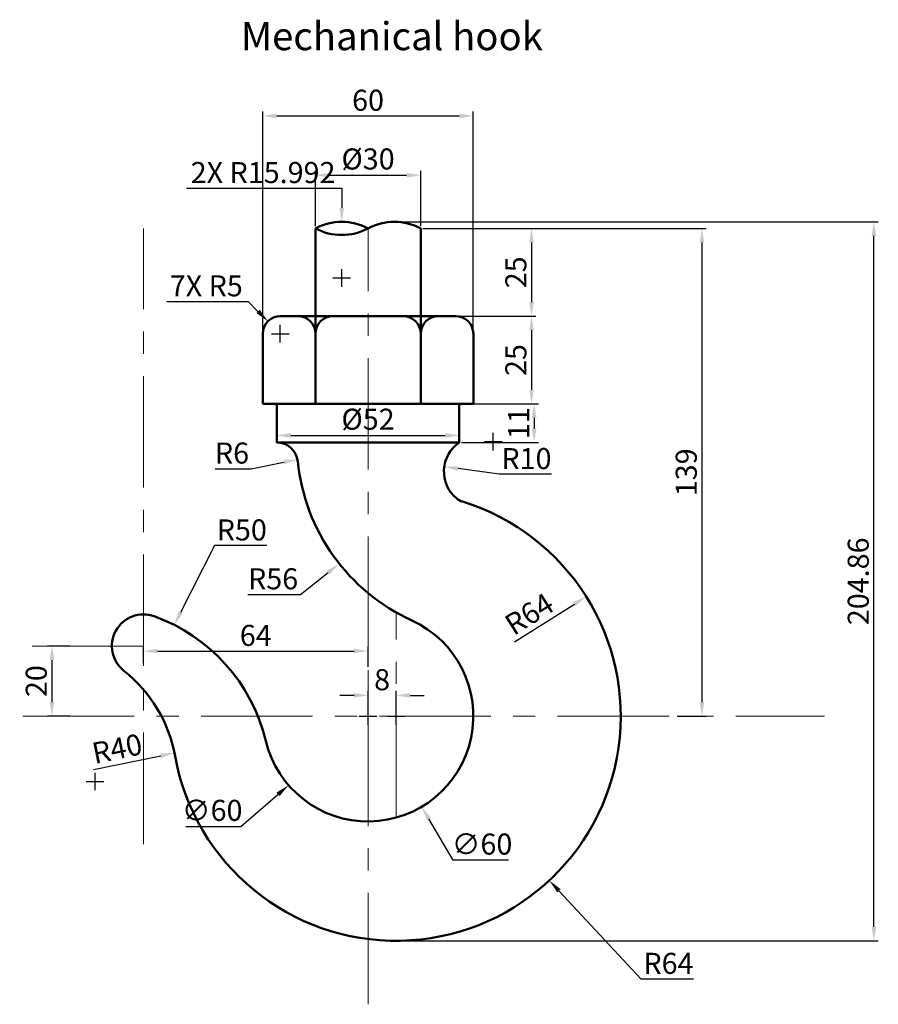
# Model space of a CAD drawing. Units: millimetres. Extents: x 42 to 286, y -15 to 266.
import ezdxf

# ---------------------------------------------------------------- set-up
doc = ezdxf.new("R2010")
doc.units = ezdxf.units.MM
doc.linetypes.add('CENTER', pattern=[50.8, 31.75, -6.35, 6.35, -6.35])
for name, color, linetype, lineweight in [('M-CNTR', 30, 'CENTER', 18), ('M-DIMS', 2, 'Continuous', 25), ('M-OUTL', 7, 'Continuous', 50), ('M-TEXT', 7, 'Continuous', 25)]:
    doc.layers.add(name, color=color, linetype=linetype, lineweight=lineweight)
doc.styles.get("Standard").update_dxf_attribs({"font": 'arial.ttf'})
doc.dimstyles.new('ISO-25', dxfattribs={"dimtxt": 6, "dimasz": 4, "dimexe": 1.25, "dimexo": 0.625, "dimtad": 1, "dimtoh": 1, "dimdec": 1, "dimtxsty": 'Standard', "dimcen": 2.5, "dimadec": 0, "dimazin": 0, "dimtfac": 1, "dimtdec": 1, "dimtofl": 0, "dimtmove": 0, "dimatfit": 3, "dimfxl": 1, "dimarcsym": 0})

# ---------------------------------------------------------------- blocks, each defined once
blk = doc.blocks.new('*D1')
at = {"layer": 'Defpoints', "color": 0, "transparency": 16777216}
for p in [(155.92, 206.24), (228.34, 67.24), (236.06, 67.24)]:
    blk.add_point(p, dxfattribs=at)
at = {"layer": 'M-DIMS', "color": 0, "lineweight": -2, "transparency": 16777216}
for p, q in [((156.55, 206.24), (237.31, 206.24)), ((236.06, 202.24), (236.06, 71.24)), ((228.97, 67.24), (237.31, 67.24))]:
    blk.add_line(p, q, dxfattribs=at)
at = {"layer": 'M-DIMS', "color": 0, "transparency": 16777216}
for points in [[(235.39, 202.24), (236.73, 202.24), (236.06, 206.24)], [(235.39, 71.24), (236.73, 71.24), (236.06, 67.24)]]:
    blk.add_solid(points, dxfattribs=at)
at = {"layer": 'M-DIMS', "color": 0, "transparency": 16777216, "insert": (232.37, 136.74), "char_height": 6, "attachment_point": 5, "rotation": 90}
blk.add_mtext('139', dxfattribs=at)
blk = doc.blocks.new('*D2')
at = {"layer": 'Defpoints', "color": 0, "transparency": 16777216}
for p in [(56.56, 87.24), (50.84, 67.24), (56.56, 67.24)]:
    blk.add_point(p, dxfattribs=at)
at = {"layer": 'M-DIMS', "color": 0, "lineweight": -2, "transparency": 16777216}
for p, q in [((55.94, 87.24), (49.59, 87.24)), ((50.84, 83.24), (50.84, 71.24)), ((55.94, 67.24), (49.59, 67.24))]:
    blk.add_line(p, q, dxfattribs=at)
at = {"layer": 'M-DIMS', "color": 0, "transparency": 16777216}
for points in [[(50.17, 83.24), (51.51, 83.24), (50.84, 87.24)], [(50.17, 71.24), (51.51, 71.24), (50.84, 67.24)]]:
    blk.add_solid(points, dxfattribs=at)
at = {"layer": 'M-DIMS', "color": 0, "transparency": 16777216, "insert": (47.15, 77.24), "char_height": 6, "attachment_point": 5, "rotation": 90}
blk.add_mtext('20', dxfattribs=at)
blk = doc.blocks.new('*D3')
at = {"layer": 'Defpoints', "color": 0, "transparency": 16777216}
for p in [(148.92, 73.18), (140.92, 67.24), (148.92, 67.24)]:
    blk.add_point(p, dxfattribs=at)
at = {"layer": 'M-DIMS', "color": 0, "lineweight": -2, "transparency": 16777216}
for p, q in [((136.92, 73.18), (132.92, 73.18)), ((140.92, 67.87), (140.92, 74.43)), ((148.92, 67.87), (148.92, 74.43)), ((152.92, 73.18), (156.92, 73.18))]:
    blk.add_line(p, q, dxfattribs=at)
at = {"layer": 'M-DIMS', "color": 0, "transparency": 16777216}
for points in [[(136.92, 73.85), (136.92, 72.52), (140.92, 73.18)], [(152.92, 73.85), (152.92, 72.52), (148.92, 73.18)]]:
    blk.add_solid(points, dxfattribs=at)
at = {"layer": 'M-DIMS', "color": 0, "transparency": 16777216, "insert": (144.92, 76.87), "char_height": 6, "attachment_point": 5}
blk.add_mtext('8', dxfattribs=at)
blk = doc.blocks.new('*D4')
at = {"layer": 'Defpoints', "color": 0, "transparency": 16777216}
for p in [(166.92, 156.24), (166.92, 145.24), (188.25, 145.24)]:
    blk.add_point(p, dxfattribs=at)
at = {"layer": 'M-DIMS', "color": 0, "lineweight": -2, "transparency": 16777216}
for p, q in [((167.55, 156.24), (189.5, 156.24)), ((188.25, 152.24), (188.25, 149.24)), ((167.55, 145.24), (189.5, 145.24))]:
    blk.add_line(p, q, dxfattribs=at)
at = {"layer": 'M-DIMS', "color": 0, "transparency": 16777216}
for points in [[(187.59, 152.24), (188.92, 152.24), (188.25, 156.24)], [(187.59, 149.24), (188.92, 149.24), (188.25, 145.24)]]:
    blk.add_solid(points, dxfattribs=at)
at = {"layer": 'M-DIMS', "color": 0, "transparency": 16777216, "insert": (184.62, 150.74), "char_height": 6, "attachment_point": 5, "rotation": 90}
blk.add_mtext('11', dxfattribs=at)
blk = doc.blocks.new('*D5')
at = {"layer": 'Defpoints', "color": 0, "transparency": 16777216}
for p in [(155.92, 181.24), (170.92, 156.24), (187.5, 156.24)]:
    blk.add_point(p, dxfattribs=at)
at = {"layer": 'M-DIMS', "color": 0, "lineweight": -2, "transparency": 16777216}
for p, q in [((156.55, 181.24), (188.75, 181.24)), ((187.5, 177.24), (187.5, 160.24)), ((171.55, 156.24), (188.75, 156.24))]:
    blk.add_line(p, q, dxfattribs=at)
at = {"layer": 'M-DIMS', "color": 0, "transparency": 16777216}
for points in [[(186.84, 177.24), (188.17, 177.24), (187.5, 181.24)], [(186.84, 160.24), (188.17, 160.24), (187.5, 156.24)]]:
    blk.add_solid(points, dxfattribs=at)
at = {"layer": 'M-DIMS', "color": 0, "transparency": 16777216, "insert": (183.82, 168.74), "char_height": 6, "attachment_point": 5, "rotation": 90}
blk.add_mtext('25', dxfattribs=at)
blk = doc.blocks.new('*D6')
at = {"layer": 'Defpoints', "color": 0, "transparency": 16777216}
for p in [(155.92, 206.24), (165.92, 181.24), (187.5, 181.24)]:
    blk.add_point(p, dxfattribs=at)
at = {"layer": 'M-DIMS', "color": 0, "lineweight": -2, "transparency": 16777216}
for p, q in [((156.55, 206.24), (188.75, 206.24)), ((187.5, 202.24), (187.5, 185.24)), ((166.55, 181.24), (188.75, 181.24))]:
    blk.add_line(p, q, dxfattribs=at)
at = {"layer": 'M-DIMS', "color": 0, "transparency": 16777216}
for points in [[(186.84, 202.24), (188.17, 202.24), (187.5, 206.24)], [(186.84, 185.24), (188.17, 185.24), (187.5, 181.24)]]:
    blk.add_solid(points, dxfattribs=at)
at = {"layer": 'M-DIMS', "color": 0, "transparency": 16777216, "insert": (183.82, 193.74), "char_height": 6, "attachment_point": 5, "rotation": 90}
blk.add_mtext('25', dxfattribs=at)
blk = doc.blocks.new('*D7')
at = {"layer": 'Defpoints', "color": 0, "transparency": 16777216}
for p in [(170.92, 238.3), (110.92, 156.24), (170.92, 156.24)]:
    blk.add_point(p, dxfattribs=at)
at = {"layer": 'M-DIMS', "color": 0, "lineweight": -2, "transparency": 16777216}
for p, q in [((110.92, 156.87), (110.92, 239.55)), ((170.92, 156.87), (170.92, 239.55)), ((114.92, 238.3), (166.92, 238.3))]:
    blk.add_line(p, q, dxfattribs=at)
at = {"layer": 'M-DIMS', "color": 0, "transparency": 16777216}
for points in [[(114.92, 238.97), (114.92, 237.63), (110.92, 238.3)], [(166.92, 238.97), (166.92, 237.63), (170.92, 238.3)]]:
    blk.add_solid(points, dxfattribs=at)
at = {"layer": 'M-DIMS', "color": 0, "transparency": 16777216, "insert": (140.92, 241.99), "char_height": 6, "attachment_point": 5}
blk.add_mtext('60', dxfattribs=at)
blk = doc.blocks.new('*D8')
at = {"layer": 'Defpoints', "color": 0, "transparency": 16777216}
for p in [(155.92, 221.41), (125.92, 206.24), (155.92, 206.24)]:
    blk.add_point(p, dxfattribs=at)
at = {"layer": 'M-DIMS', "color": 0, "lineweight": -2, "transparency": 16777216}
for p, q in [((125.92, 206.87), (125.92, 222.66)), ((155.92, 206.87), (155.92, 222.66)), ((129.92, 221.41), (151.92, 221.41))]:
    blk.add_line(p, q, dxfattribs=at)
at = {"layer": 'M-DIMS', "color": 0, "transparency": 16777216}
for points in [[(129.92, 222.07), (129.92, 220.74), (125.92, 221.41)], [(151.92, 222.07), (151.92, 220.74), (155.92, 221.41)]]:
    blk.add_solid(points, dxfattribs=at)
at = {"layer": 'M-DIMS', "color": 0, "transparency": 16777216, "insert": (140.92, 225.26), "char_height": 6, "attachment_point": 5}
blk.add_mtext('%%C30', dxfattribs=at)
blk = doc.blocks.new('*D9')
at = {"layer": 'Defpoints', "color": 0, "transparency": 16777216}
for p in [(114.92, 150.74), (166.92, 150.74), (166.92, 147.25)]:
    blk.add_point(p, dxfattribs=at)
at = {"layer": 'M-DIMS', "color": 0, "lineweight": -2, "transparency": 16777216}
for p, q in [((114.92, 150.12), (114.92, 146)), ((166.92, 150.12), (166.92, 146)), ((118.92, 147.25), (162.92, 147.25))]:
    blk.add_line(p, q, dxfattribs=at)
at = {"layer": 'M-DIMS', "color": 0, "transparency": 16777216}
for points in [[(118.92, 147.92), (118.92, 146.58), (114.92, 147.25)], [(162.92, 147.92), (162.92, 146.58), (166.92, 147.25)]]:
    blk.add_solid(points, dxfattribs=at)
at = {"layer": 'M-DIMS', "color": 0, "transparency": 16777216, "insert": (140.92, 151.1), "char_height": 6, "attachment_point": 5}
blk.add_mtext('%%C52', dxfattribs=at)
blk = doc.blocks.new('*D10')
at = {"layer": 'Defpoints', "color": 0, "transparency": 16777216}
for p in [(120.8, 140.43), (114.92, 139.24)]:
    blk.add_point(p, dxfattribs=at)
at = {"layer": 'M-DIMS', "color": 0, "lineweight": -2, "transparency": 16777216}
for p, q in [((97.31, 137.76), (107.61, 137.76)), ((107.61, 137.76), (116.88, 139.64))]:
    blk.add_line(p, q, dxfattribs=at)
at = {"layer": 'M-DIMS', "color": 0, "transparency": 16777216}
blk.add_solid([(116.75, 140.29), (117.02, 138.98), (120.8, 140.43)], dxfattribs=at)
at = {"layer": 'M-DIMS', "color": 0, "transparency": 16777216, "insert": (102.15, 141.45), "char_height": 6, "attachment_point": 5}
blk.add_mtext('R6', dxfattribs=at)
blk = doc.blocks.new('*D11')
at = {"layer": 'Defpoints', "color": 0, "transparency": 16777216}
for p in [(162.64, 138.34), (172.54, 136.98)]:
    blk.add_point(p, dxfattribs=at)
at = {"layer": 'M-DIMS', "color": 0, "lineweight": -2, "transparency": 16777216}
for p, q in [((178.27, 136.2), (166.6, 137.8)), ((193.21, 136.2), (178.27, 136.2))]:
    blk.add_line(p, q, dxfattribs=at)
at = {"layer": 'M-DIMS', "color": 0, "transparency": 16777216}
blk.add_solid([(166.69, 138.46), (166.51, 137.14), (162.64, 138.34)], dxfattribs=at)
at = {"layer": 'M-DIMS', "color": 0, "transparency": 16777216, "insert": (186.06, 139.88), "char_height": 6, "attachment_point": 5}
blk.add_mtext('R10', dxfattribs=at)
blk = doc.blocks.new('*D12')
at = {"layer": 'Defpoints', "color": 0, "transparency": 16777216}
for p in [(176.61, 145.49), (132.72, 110.7)]:
    blk.add_point(p, dxfattribs=at)
at = {"layer": 'M-DIMS', "color": 0, "lineweight": -2, "transparency": 16777216}
for p, q in [((176.61, 142.99), (176.61, 147.99)), ((174.11, 145.49), (179.11, 145.49)), ((121.65, 101.93), (129.59, 108.22)), ((106.69, 101.93), (121.65, 101.93))]:
    blk.add_line(p, q, dxfattribs=at)
at = {"layer": 'M-DIMS', "color": 0, "transparency": 16777216}
blk.add_solid([(129.17, 108.74), (130, 107.7), (132.72, 110.7)], dxfattribs=at)
at = {"layer": 'M-DIMS', "color": 0, "transparency": 16777216, "insert": (113.86, 105.62), "char_height": 6, "attachment_point": 5}
blk.add_mtext('R56', dxfattribs=at)
blk = doc.blocks.new('*D13')
at = {"layer": 'Defpoints', "color": 0, "transparency": 16777216}
for p in [(203.09, 101.33), (148.92, 67.24)]:
    blk.add_point(p, dxfattribs=at)
at = {"layer": 'M-DIMS', "color": 0, "lineweight": -2, "transparency": 16777216}
blk.add_line((182.65, 88.46), (199.71, 99.2), dxfattribs=at)
at = {"layer": 'M-DIMS', "color": 0, "transparency": 16777216}
blk.add_solid([(199.35, 99.76), (200.06, 98.63), (203.09, 101.33)], dxfattribs=at)
at = {"layer": 'M-DIMS', "color": 0, "transparency": 16777216, "insert": (187.27, 95.73), "char_height": 6, "attachment_point": 5, "rotation": 32.1817}
blk.add_mtext('R64', dxfattribs=at)
blk = doc.blocks.new('*D14')
at = {"layer": 'Defpoints', "color": 0, "transparency": 16777216}
for p in [(85.77, 56.79), (46.58, 48.77)]:
    blk.add_point(p, dxfattribs=at)
at = {"layer": 'M-DIMS', "color": 0, "lineweight": -2, "transparency": 16777216}
blk.add_line((62.68, 52.06), (81.85, 55.98), dxfattribs=at)
at = {"layer": 'M-DIMS', "color": 0, "transparency": 16777216}
blk.add_solid([(81.71, 56.64), (81.98, 55.33), (85.77, 56.79)], dxfattribs=at)
at = {"layer": 'M-DIMS', "color": 0, "transparency": 16777216, "insert": (69.56, 57.24), "char_height": 6, "attachment_point": 5, "rotation": 11.5627}
blk.add_mtext('R40', dxfattribs=at)
blk = doc.blocks.new('*D15')
at = {"layer": 'Defpoints', "color": 0, "transparency": 16777216}
for p in [(85.7, 93.24), (63.12, 48.64)]:
    blk.add_point(p, dxfattribs=at)
at = {"layer": 'M-DIMS', "color": 0, "lineweight": -2, "transparency": 16777216}
for p, q in [((97.15, 115.86), (87.51, 96.81)), ((112.09, 115.86), (97.15, 115.86)), ((63.12, 46.14), (63.12, 51.14)), ((60.62, 48.64), (65.62, 48.64))]:
    blk.add_line(p, q, dxfattribs=at)
at = {"layer": 'M-DIMS', "color": 0, "transparency": 16777216}
blk.add_solid([(86.91, 97.11), (88.1, 96.51), (85.7, 93.24)], dxfattribs=at)
at = {"layer": 'M-DIMS', "color": 0, "transparency": 16777216, "insert": (104.94, 119.55), "char_height": 6, "attachment_point": 5}
blk.add_mtext('R50', dxfattribs=at)
blk = doc.blocks.new('*D16')
at = {"layer": 'Defpoints', "color": 0, "transparency": 16777216}
for p in [(125.65, 93.06), (156.2, 41.42)]:
    blk.add_point(p, dxfattribs=at)
at = {"layer": 'M-DIMS', "color": 0, "lineweight": -2, "transparency": 16777216}
for p, q in [((140.92, 64.74), (140.92, 69.74)), ((138.42, 67.24), (143.42, 67.24)), ((165.22, 26.17), (158.24, 37.98)), ((180.95, 26.17), (165.22, 26.17))]:
    blk.add_line(p, q, dxfattribs=at)
at = {"layer": 'M-DIMS', "color": 0, "transparency": 16777216}
blk.add_solid([(158.81, 38.32), (157.66, 37.64), (156.2, 41.42)], dxfattribs=at)
at = {"layer": 'M-DIMS', "color": 0, "transparency": 16777216, "insert": (173.4, 30.03), "char_height": 6, "attachment_point": 5}
blk.add_mtext('∅60', dxfattribs=at)
blk = doc.blocks.new('*D17')
at = {"layer": 'Defpoints', "color": 0, "transparency": 16777216}
for p in [(140.92, 85.8), (76.92, 81.77), (140.92, 80.64)]:
    blk.add_point(p, dxfattribs=at)
at = {"layer": 'M-DIMS', "color": 0, "lineweight": -2, "transparency": 16777216}
for p, q in [((76.92, 82.4), (76.92, 87.05)), ((140.92, 81.27), (140.92, 87.05)), ((80.92, 85.8), (136.92, 85.8))]:
    blk.add_line(p, q, dxfattribs=at)
at = {"layer": 'M-DIMS', "color": 0, "transparency": 16777216}
for points in [[(80.92, 86.47), (80.92, 85.14), (76.92, 85.8)], [(136.92, 86.47), (136.92, 85.14), (140.92, 85.8)]]:
    blk.add_solid(points, dxfattribs=at)
at = {"layer": 'M-DIMS', "color": 0, "transparency": 16777216, "insert": (108.92, 89.49), "char_height": 6, "attachment_point": 5}
blk.add_mtext('64', dxfattribs=at)
blk = doc.blocks.new('*D18')
at = {"layer": 'Defpoints', "color": 0, "transparency": 16777216}
for p in [(148.42, 208.11), (285.08, 208.11), (150.14, 3.25)]:
    blk.add_point(p, dxfattribs=at)
at = {"layer": 'M-DIMS', "color": 0, "lineweight": -2, "transparency": 16777216}
for p, q in [((149.05, 208.11), (286.33, 208.11)), ((285.08, 7.25), (285.08, 204.11)), ((150.76, 3.25), (286.33, 3.25))]:
    blk.add_line(p, q, dxfattribs=at)
at = {"layer": 'M-DIMS', "color": 0, "transparency": 16777216}
for points in [[(284.41, 204.11), (285.74, 204.11), (285.08, 208.11)], [(284.41, 7.25), (285.74, 7.25), (285.08, 3.25)]]:
    blk.add_solid(points, dxfattribs=at)
at = {"layer": 'M-DIMS', "color": 0, "transparency": 16777216, "insert": (281.39, 105.68), "char_height": 6, "attachment_point": 5, "rotation": 90}
blk.add_mtext('204.86', dxfattribs=at)
blk = doc.blocks.new('*D19')
at = {"layer": 'Defpoints', "color": 0, "transparency": 16777216}
for p in [(148.92, 67.24), (192.57, 20.43)]:
    blk.add_point(p, dxfattribs=at)
at = {"layer": 'M-DIMS', "color": 0, "lineweight": -2, "transparency": 16777216}
for p, q in [((148.92, 64.74), (148.92, 69.74)), ((146.42, 67.24), (151.42, 67.24)), ((218.75, -7.66), (195.29, 17.5)), ((233.69, -7.66), (218.75, -7.66))]:
    blk.add_line(p, q, dxfattribs=at)
at = {"layer": 'M-DIMS', "color": 0, "transparency": 16777216}
blk.add_solid([(195.78, 17.96), (194.81, 17.05), (192.57, 20.43)], dxfattribs=at)
at = {"layer": 'M-DIMS', "color": 0, "transparency": 16777216, "insert": (226.53, -3.97), "char_height": 6, "attachment_point": 5}
blk.add_mtext('R64', dxfattribs=at)
blk = doc.blocks.new('*D20')
at = {"layer": 'Defpoints', "color": 0, "transparency": 16777216}
for p in [(163.58, 86.91), (118.27, 47.57)]:
    blk.add_point(p, dxfattribs=at)
at = {"layer": 'M-DIMS', "color": 0, "lineweight": -2, "transparency": 16777216}
for p, q in [((140.92, 64.74), (140.92, 69.74)), ((138.42, 67.24), (143.42, 67.24)), ((104.68, 35.77), (115.25, 44.95)), ((88.95, 35.77), (104.68, 35.77))]:
    blk.add_line(p, q, dxfattribs=at)
at = {"layer": 'M-DIMS', "color": 0, "transparency": 16777216}
blk.add_solid([(114.81, 45.45), (115.69, 44.45), (118.27, 47.57)], dxfattribs=at)
at = {"layer": 'M-DIMS', "color": 0, "transparency": 16777216, "insert": (96.5, 39.63), "char_height": 6, "attachment_point": 5}
blk.add_mtext('∅60', dxfattribs=at)
blk = doc.blocks.new('*D21')
at = {"layer": 'Defpoints', "color": 0, "transparency": 16777216}
for p in [(133.42, 208.11), (133.42, 192.12)]:
    blk.add_point(p, dxfattribs=at)
at = {"layer": 'M-DIMS', "color": 0, "lineweight": -2, "transparency": 16777216}
for p, q in [((89.21, 217.7), (133.42, 217.7)), ((133.42, 217.7), (133.42, 212.11)), ((133.42, 189.62), (133.42, 194.62)), ((130.92, 192.12), (135.92, 192.12))]:
    blk.add_line(p, q, dxfattribs=at)
at = {"layer": 'M-DIMS', "color": 0, "transparency": 16777216}
blk.add_solid([(134.09, 212.11), (132.76, 212.11), (133.42, 208.11)], dxfattribs=at)
at = {"layer": 'M-DIMS', "color": 0, "transparency": 16777216, "insert": (111.01, 221.39), "char_height": 6, "attachment_point": 5}
blk.add_mtext('2X R15.992', dxfattribs=at)
blk = doc.blocks.new('*D22')
at = {"layer": 'Defpoints', "color": 0, "transparency": 16777216}
for p in [(112.39, 179.78), (115.92, 176.24)]:
    blk.add_point(p, dxfattribs=at)
at = {"layer": 'M-DIMS', "color": 0, "lineweight": -2, "transparency": 16777216}
for p, q in [((83.54, 185.43), (106.73, 185.43)), ((106.73, 185.43), (109.56, 182.6)), ((115.92, 173.74), (115.92, 178.74)), ((113.42, 176.24), (118.42, 176.24))]:
    blk.add_line(p, q, dxfattribs=at)
at = {"layer": 'M-DIMS', "color": 0, "transparency": 16777216}
blk.add_solid([(110.03, 183.08), (109.09, 182.13), (112.39, 179.78)], dxfattribs=at)
at = {"layer": 'M-DIMS', "color": 0, "transparency": 16777216, "insert": (94.82, 189.11), "char_height": 6, "attachment_point": 5}
blk.add_mtext('7X R5', dxfattribs=at)

msp = doc.modelspace()

# ---------------------------------------------------------------- linework, layer by layer
at = {"layer": 'M-CNTR'}
for p, q in [((76.9233, 30.8034), (76.9233, 206.2406)), ((140.9233, -14.8615), (140.9233, 206.2406)), ((148.9233, 38.327), (148.9233, 96.8096)), ((76.9233, 87.2406), (41.6504, 87.2406)), ((42.5381, 67.2406), (270.977, 67.2406))]:
    msp.add_line(p, q, dxfattribs=at)
at = {"layer": 'M-OUTL'}
for p, q in [((125.9233, 156.2406), (125.9233, 206.2406)), ((155.9233, 206.2406), (155.9233, 156.2406)), ((115.9233, 181.2406), (165.9233, 181.2406)), ((110.9233, 156.2406), (110.9233, 176.2406)), ((170.9233, 176.2406), (170.9233, 156.2406)), ((170.9233, 156.2406), (110.9233, 156.2406))]:
    msp.add_line(p, q, dxfattribs=at)
msp.add_lwpolyline([(114.9233, 156.2406), (166.9233, 156.2406), (166.9233, 145.2406), (114.9233, 145.2406)], close=True, dxfattribs=at)
for centre, radius, start, end in [((133.4233, 192.1163), 15.9921, 62.031765, 117.968235), ((148.4233, 192.1163), 15.9921, 62.031765, 117.968235), ((133.4233, 220.365), 15.9921, 242.031765, 297.968235), ((115.9233, 176.2406), 5, 90, 180), ((120.9233, 176.2406), 5, 0, 90), ((130.9233, 176.2406), 5, 90, 180), ((150.9233, 176.2406), 5, 0, 90), ((160.9233, 176.2406), 5, 90, 180), ((165.9233, 176.2406), 5, 0, 90), ((114.9233, 139.2406), 6, 5.78298, 90), ((172.5438, 136.9808), 10, 124.197644, 229.903617), ((176.6078, 145.4878), 56, 185.78298, 245.484738), ((169.3234, 133.156), 5, 229.903617, 252.80325), ((148.9233, 67.2406), 64, 190.230905, 72.80325), ((76.9233, 87.2406), 9, 70.321528, 231.733931), ((63.1169, 48.6351), 50, 13.448339, 70.321528), ((140.9233, 67.2406), 30, 193.448339, 65.484738), ((46.5769, 48.7686), 40, 10.230905, 51.733931)]:
    msp.add_arc(centre, radius, start, end, dxfattribs=at)

# ---------------------------------------------------------------- texts
at = {"layer": 'M-TEXT', "insert": (104.7025, 265.0387), "char_height": 8, "attachment_point": 1}
msp.add_mtext_dynamic_manual_height_columns('Mechanical hook', width=86.743585, gutter_width=12.5, heights=[0], dxfattribs=at)

# ---------------------------------------------------------------- dimensions: what is measured, and where the dimension line sits
at = {"layer": 'M-DIMS'}
for base, p1, p2, picture, middle in [((170.9233, 238.2993), (110.9233, 156.2406), (170.9233, 156.2406), '*D7', (140.9233, 241.9877)), ((140.9233, 85.8037), (76.9233, 81.7723), (140.9233, 80.6435), '*D17', (108.9233, 89.4921)), ((148.9233, 73.1818), (140.9233, 67.2406), (148.9233, 67.2406), '*D3', (144.9233, 76.8702))]:
    dim = msp.add_linear_dim(base=base, p1=p1, p2=p2, dimstyle='ISO-25', override={"dimclrd": 0, "dimclre": 0, "dimclrt": 0}, dxfattribs=at)
    dim.commit()
    dim.dimension.update_dxf_attribs({"geometry": picture, "text_midpoint": middle})
dim = msp.add_radius_dim(center=(133.4233, 192.1163), mpoint=(133.423, 208.1084), text='2X <>', dimstyle='ISO-25', override={"dimdec": 3, "dimlfac": 1, "dimrnd": 0, "dimzin": 0, "dimdsep": 46, "dimlunit": 2}, dxfattribs=at)
dim.commit()
dim.dimension.update_dxf_attribs({"geometry": '*D21', "text_midpoint": (111.0059, 217.7036), "dimtype": 164})
for base, p1, p2, picture, middle in [((155.9233, 221.4064), (125.9233, 206.2406), (155.9233, 206.2406), '*D8', (140.9233, 225.2627)), ((166.9233, 147.2487), (114.9233, 150.7406), (166.9233, 150.7406), '*D9', (140.9233, 151.1049))]:
    dim = msp.add_linear_dim(base=base, p1=p1, p2=p2, text='%%C<>', dimstyle='ISO-25', override={"dimclrd": 0, "dimclre": 0, "dimclrt": 0}, dxfattribs=at)
    dim.commit()
    dim.dimension.update_dxf_attribs({"geometry": picture, "text_midpoint": middle})
for base, p1, p2, override, picture, middle in [((285.077, 208.1084), (150.1389, 3.2522), (148.4233, 208.1084), {"dimdec": 2, "dimlfac": 1, "dimrnd": 0, "dimzin": 0, "dimdsep": 46, "dimlunit": 2}, '*D18', (281.3886, 105.6803)), ((236.0601, 67.2406), (155.9233, 206.2406), (228.3402, 67.2406), {"dimclrd": 0, "dimclre": 0, "dimclrt": 0}, '*D1', (232.3696, 136.7406)), ((187.5039, 181.2406), (155.9233, 206.2406), (165.9233, 181.2406), {"dimclrd": 0, "dimclre": 0, "dimclrt": 0}, '*D6', (183.8155, 193.7406)), ((187.5039, 156.2406), (155.9233, 181.2406), (170.9233, 156.2406), {"dimclrd": 0, "dimclre": 0, "dimclrt": 0}, '*D5', (183.8155, 168.7406)), ((188.2524, 145.2406), (166.9233, 156.2406), (166.9233, 145.2406), {"dimclrd": 0, "dimclre": 0, "dimclrt": 0}, '*D4', (184.6151, 150.7406)), ((50.8409, 67.2406), (56.5613, 87.2406), (56.5613, 67.2406), {"dimclrd": 0, "dimclre": 0, "dimclrt": 0}, '*D2', (47.1525, 77.2406))]:
    dim = msp.add_linear_dim(base=base, p1=p1, p2=p2, angle=90, dimstyle='ISO-25', override=override, dxfattribs=at)
    dim.commit()
    dim.dimension.update_dxf_attribs({"geometry": picture, "text_midpoint": middle})
dim = msp.add_radius_dim(center=(115.9233, 176.2406), mpoint=(112.3878, 179.7762), text='7X <>', dimstyle='ISO-25', override={"dimdec": 0, "dimlfac": 1, "dimrnd": 0, "dimzin": 0, "dimdsep": 46, "dimlunit": 2}, dxfattribs=at)
dim.commit()
dim.dimension.update_dxf_attribs({"geometry": '*D22', "text_midpoint": (94.8243, 189.1093)})
dim = msp.add_radius_dim(center=(176.6078, 145.4878), mpoint=(132.7215, 110.7028), dimstyle='ISO-25', override={"dimclrd": 0, "dimclre": 0, "dimclrt": 0}, dxfattribs=at)
dim.commit()
dim.dimension.update_dxf_attribs({"geometry": '*D12', "text_midpoint": (113.8591, 105.6162)})
for center, mpoint, override, picture, middle in [((114.9233, 139.2406), (120.8047, 140.4277), {"dimclrd": 0, "dimclre": 0, "dimclrt": 0}, '*D10', (107.6102, 137.7645)), ((172.5438, 136.9808), (162.6365, 138.3395), {"dimclrd": 0, "dimclre": 0, "dimclrt": 0}, '*D11', (178.2734, 136.195)), ((63.1169, 48.6351), (85.7014, 93.2439), {"dimclrd": 0, "dimclre": 0, "dimclrt": 0}, '*D15', (104.9367, 115.8638)), ((148.9233, 67.2406), (203.0905, 101.3274), {"dimclrd": 0, "dimclre": 0, "dimclrt": 0}, '*D13', (189.2342, 92.6078)), ((148.9233, 67.2406), (192.566, 20.4292), {"dimdec": 0, "dimlfac": 1, "dimrnd": 0, "dimzin": 0, "dimdsep": 46, "dimlunit": 2}, '*D19', (226.5329, -7.6577)), ((46.5769, 48.7686), (85.7652, 56.7862), {"dimclrd": 0, "dimclre": 0, "dimclrt": 0}, '*D14', (70.3022, 53.6226))]:
    dim = msp.add_radius_dim(center=center, mpoint=mpoint, dimstyle='ISO-25', override=override, dxfattribs=at)
    dim.commit()
    dim.dimension.update_dxf_attribs({"geometry": picture, "text_midpoint": middle, "dimtype": 164})
for p1, p2, override, picture, middle in [((125.6464, 93.0595), (156.2002, 41.4217), {"dimclrd": 0, "dimclre": 0, "dimclrt": 0}, '*D16', (173.4011, 26.1693)), ((163.5773, 86.9078), (118.2694, 47.5734), {"dimdec": 0, "dimlfac": 1, "dimrnd": 0, "dimzin": 0, "dimdsep": 46, "dimlunit": 2}, '*D20', (96.5009, 35.7731))]:
    dim = msp.add_diameter_dim_2p(p1=p1, p2=p2, dimstyle='ISO-25', override=override, dxfattribs=at)
    dim.commit()
    dim.dimension.update_dxf_attribs({"geometry": picture, "text_midpoint": middle, "dimtype": 163})

doc.saveas('drawing.dxf')
